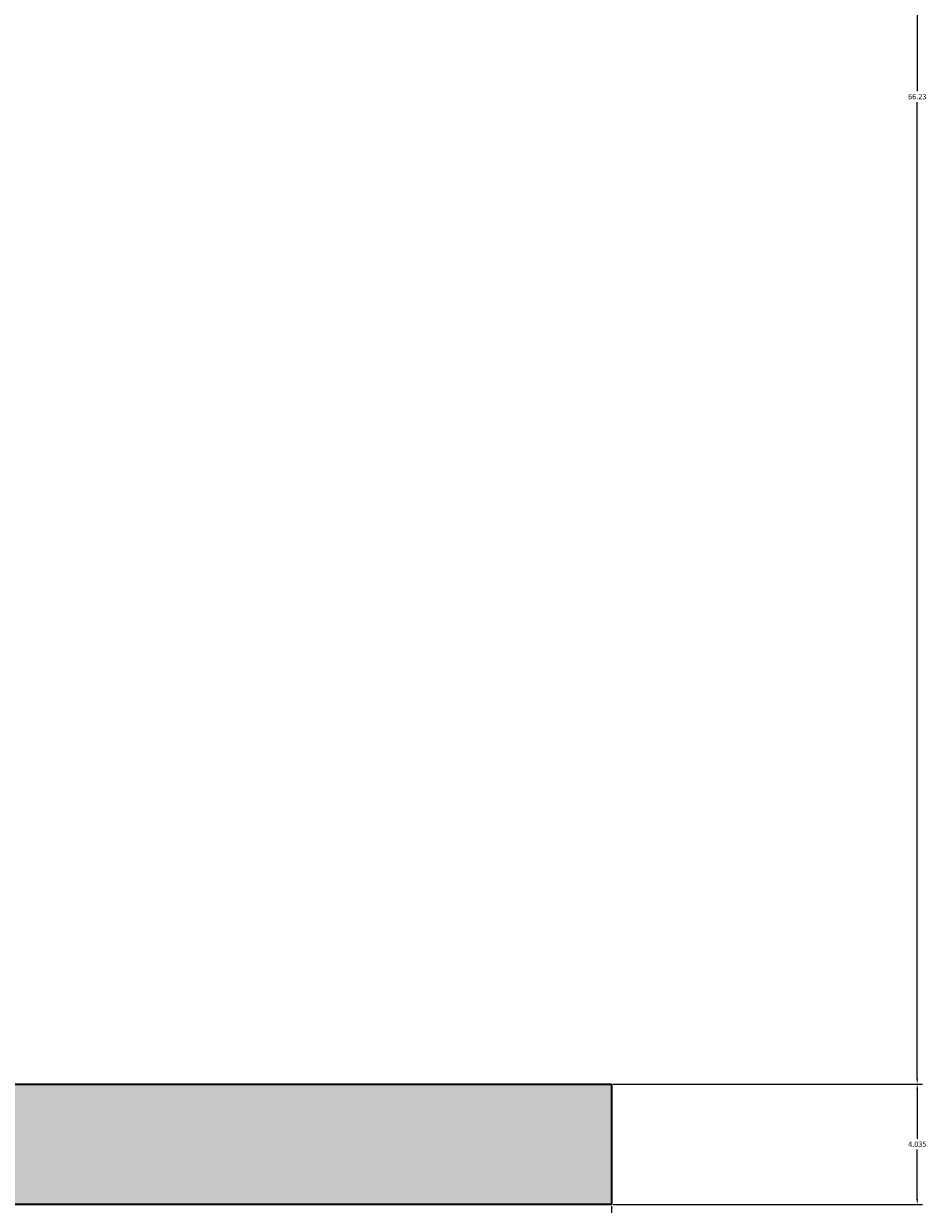
# Model space of a CAD drawing. Units: millimetres. Extents: x 446512 to 447461, y 70395 to 70610.
# Tile 37 of 39: x 447431 to 447461, y 70432 to 70472. Entities that reach past the tile are written whole.
import ezdxf

# ---------------------------------------------------------------- set-up
doc = ezdxf.new("R2010")
doc.units = ezdxf.units.MM
for name, color, linetype, lineweight in [('A-ANNO-DIMS', 2, 'Continuous', 18), ('A-FURN', 7, 'Continuous', 35), ('A-FURN-PATT', 38, 'Continuous', 13)]:
    doc.layers.add(name, color=color, linetype=linetype, lineweight=lineweight)
doc.styles.get("Standard").update_dxf_attribs({"font": 'arial.ttf'})
doc.dimstyles.get("Standard").update_dxf_attribs({"dimtxt": 0.18, "dimasz": 0.18, "dimexe": 0.18, "dimexo": 0.0625, "dimgap": 0.09, "dimtad": 0, "dimtih": 1, "dimtoh": 1, "dimdec": 4, "dimzin": 0, "dimdsep": 46, "dimtxsty": 'Standard', "dimcen": 0.09, "dimadec": 0, "dimazin": 0, "dimtfac": 1, "dimtdec": 4, "dimtofl": 0, "dimtmove": 0, "dimatfit": 3, "dimfxl": 1, "dimtolj": 1, "dimtzin": 0, "dimarcsym": 0})

# ---------------------------------------------------------------- blocks, each defined once
blk = doc.blocks.new('*D61')
at = {"layer": 'A-ANNO-DIMS', "color": 0, "lineweight": -2, "transparency": 16777216}
for p, q in [((447254.943, 70452.792), (447254.943, 70394.885)), ((447450.532, 70432.19), (447450.532, 70394.885)), ((447255.123, 70395.065), (447352.352, 70395.065)), ((447450.352, 70395.065), (447353.122, 70395.065))]:
    blk.add_line(p, q, dxfattribs=at)
at = {"layer": 'A-ANNO-DIMS', "color": 0, "transparency": 16777216}
for points in [[(447255.123, 70395.095), (447255.123, 70395.035), (447254.943, 70395.065)], [(447450.352, 70395.095), (447450.352, 70395.035), (447450.532, 70395.065)]]:
    blk.add_solid(points, dxfattribs=at)
at = {"layer": 'Defpoints', "color": 0, "transparency": 16777216}
for p in [(447254.943, 70452.855), (447450.532, 70432.253), (447450.532, 70395.065)]:
    blk.add_point(p, dxfattribs=at)
at = {"layer": 'A-ANNO-DIMS', "color": 0, "transparency": 16777216, "insert": (447352.737, 70395.065), "char_height": 0.18, "attachment_point": 5}
blk.add_mtext('\\A1;195.6', dxfattribs=at)
blk = doc.blocks.new('*D68')
at = {"layer": 'A-ANNO-DIMS', "color": 0, "lineweight": -2, "transparency": 16777216}
for p, q in [((447450.594, 70436.288), (447460.962, 70436.288)), ((447460.782, 70436.108), (447460.782, 70434.452)), ((447460.782, 70432.433), (447460.782, 70434.088)), ((447450.594, 70432.253), (447460.962, 70432.253))]:
    blk.add_line(p, q, dxfattribs=at)
at = {"layer": 'A-ANNO-DIMS', "color": 0, "transparency": 16777216}
for points in [[(447460.752, 70436.108), (447460.812, 70436.108), (447460.782, 70436.288)], [(447460.752, 70432.433), (447460.812, 70432.433), (447460.782, 70432.253)]]:
    blk.add_solid(points, dxfattribs=at)
at = {"layer": 'Defpoints', "color": 0, "transparency": 16777216}
for p in [(447450.532, 70436.288), (447460.782, 70436.288), (447450.532, 70432.253)]:
    blk.add_point(p, dxfattribs=at)
at = {"layer": 'A-ANNO-DIMS', "color": 0, "transparency": 16777216, "insert": (447460.782, 70434.27), "char_height": 0.18, "attachment_point": 5}
blk.add_mtext('\\A1;4.035', dxfattribs=at)
blk = doc.blocks.new('*D69')
at = {"layer": 'A-ANNO-DIMS', "color": 0, "lineweight": -2, "transparency": 16777216}
for p, q in [((447450.594, 70502.515), (447460.962, 70502.515)), ((447460.782, 70502.335), (447460.782, 70469.583)), ((447460.782, 70436.468), (447460.782, 70469.219)), ((447450.594, 70436.288), (447460.962, 70436.288))]:
    blk.add_line(p, q, dxfattribs=at)
at = {"layer": 'A-ANNO-DIMS', "color": 0, "transparency": 16777216}
for points in [[(447460.752, 70502.335), (447460.812, 70502.335), (447460.782, 70502.515)], [(447460.752, 70436.468), (447460.812, 70436.468), (447460.782, 70436.288)]]:
    blk.add_solid(points, dxfattribs=at)
at = {"layer": 'Defpoints', "color": 0, "transparency": 16777216}
for p in [(447450.532, 70502.515), (447460.782, 70502.515), (447450.532, 70436.288)]:
    blk.add_point(p, dxfattribs=at)
at = {"layer": 'A-ANNO-DIMS', "color": 0, "transparency": 16777216, "insert": (447460.782, 70469.401), "char_height": 0.18, "attachment_point": 5}
blk.add_mtext('\\A1;66.23', dxfattribs=at)

msp = doc.modelspace()

# ---------------------------------------------------------------- hatches: boundary and pattern name
at = {"layer": 'A-FURN-PATT'}
h = msp.add_hatch(color=256, dxfattribs=at)
h.dxf.hatch_style = 1
h.paths.add_polyline_path([(447365.4251, 70432.2526), (447365.4251, 70436.2876), (447340.0494, 70436.2876), (447340.0494, 70432.2526)])
h.paths.add_polyline_path([(447426.0142, 70436.2876), (447426.0142, 70432.2526), (447450.5318, 70432.2526), (447450.5318, 70436.2876)])

# ---------------------------------------------------------------- linework, layer by layer
at = {"layer": 'A-FURN'}
msp.add_lwpolyline([(447340.0494, 70436.2876), (447450.5318, 70436.2876), (447450.5318, 70432.2526), (447340.0494, 70432.2526)], close=True, dxfattribs=at)

# ---------------------------------------------------------------- dimensions: what is measured, and where the dimension line sits
at = {"layer": 'A-ANNO-DIMS'}
for base, p1, p2, override, picture, middle in [((447460.7818, 70502.5146), (447450.5318, 70436.2876), (447450.5318, 70502.5146), {"dimdec": 2, "dimlfac": 1, "dimrnd": 0, "dimzin": 0, "dimdsep": 46, "dimlunit": 2}, '*D69', (447460.7818, 70469.4011)), ((447460.7818, 70436.2876), (447450.5318, 70432.2526), (447450.5318, 70436.2876), {"dimdec": 3, "dimlfac": 1, "dimrnd": 0, "dimzin": 0, "dimdsep": 46, "dimlunit": 2}, '*D68', (447460.7818, 70434.2701))]:
    dim = msp.add_linear_dim(base=base, p1=p1, p2=p2, angle=90, dimstyle='Standard', override=override, dxfattribs=at)
    dim.commit()
    dim.dimension.update_dxf_attribs({"geometry": picture, "text_midpoint": middle})
dim = msp.add_linear_dim(base=(447450.5318, 70395.0645), p1=(447254.9427, 70452.855), p2=(447450.5318, 70432.2526), dimstyle='Standard', override={"dimdec": 1, "dimlfac": 1, "dimrnd": 0, "dimzin": 0, "dimdsep": 46, "dimlunit": 2}, dxfattribs=at)
dim.commit()
dim.dimension.update_dxf_attribs({"geometry": '*D61', "text_midpoint": (447352.7372, 70395.0645)})

doc.saveas('drawing.dxf')
